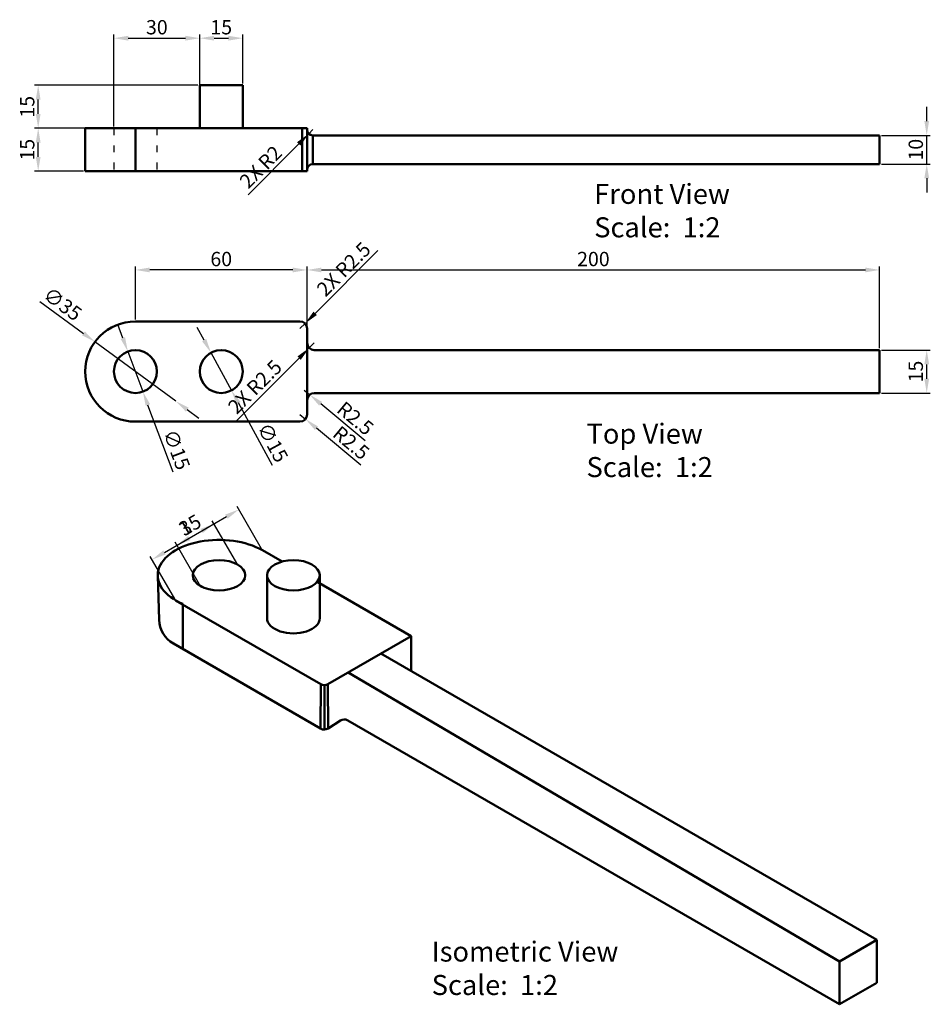
# Model space of a CAD drawing. Units: millimetres. Extents: x 2577 to 3382, y -259 to 299.
# Tile 2 of 2: x 3064 to 3382, y -124 to 220. Entities that reach past the tile are written whole.
import ezdxf

# ---------------------------------------------------------------- set-up
doc = ezdxf.new("R2010")
doc.units = ezdxf.units.MM
doc.linetypes.add('ACAD_ISO03W100', pattern=[30, 12, -18])
for name, color, linetype, lineweight in [('M-DIMS', 2, 'Continuous', 25), ('M-HIDN', 7, 'ACAD_ISO03W100', 25), ('M-OUTL', 7, 'Continuous', 50), ('M-TEXT', 7, 'Continuous', 25)]:
    doc.layers.add(name, color=color, linetype=linetype, lineweight=lineweight)
doc.styles.get("Standard").update_dxf_attribs({"font": 'arial.ttf'})
doc.dimstyles.new('ISO-25', dxfattribs={"dimtxt": 5, "dimasz": 5, "dimexe": 1.25, "dimexo": 0.625, "dimtad": 1, "dimdec": 0, "dimtxsty": 'Standard', "dimcen": 2.5, "dimadec": 0, "dimazin": 0, "dimtfac": 1, "dimtdec": 0, "dimtmove": 0, "dimatfit": 3, "dimfxl": 1, "dimarcsym": 0})

# ---------------------------------------------------------------- blocks, each defined once
blk = doc.blocks.new('*D12')
at = {"layer": 'Defpoints', "color": 0, "transparency": 16777216}
for p in [(3090.35, 107.42), (3118.56, 86.7)]:
    blk.add_point(p, dxfattribs=at)
at = {"layer": 'M-DIMS', "color": 0, "lineweight": -2, "transparency": 16777216}
for p, q in [((3071.1, 121.56), (3086.32, 110.38)), ((3118.56, 86.7), (3090.35, 107.42)), ((3122.59, 83.74), (3126.62, 80.78))]:
    blk.add_line(p, q, dxfattribs=at)
at = {"layer": 'M-DIMS', "color": 0, "transparency": 16777216}
for points in [[(3086.81, 111.05), (3085.83, 109.71), (3090.35, 107.42)], [(3123.08, 84.41), (3122.1, 83.07), (3118.56, 86.7)]]:
    blk.add_solid(points, dxfattribs=at)
at = {"layer": 'M-DIMS', "color": 0, "transparency": 16777216, "insert": (3078.66, 120.12), "char_height": 5, "attachment_point": 5, "rotation": 323.7034}
blk.add_mtext('∅35', dxfattribs=at)
blk = doc.blocks.new('*D13')
at = {"layer": 'Defpoints', "color": 0, "transparency": 16777216}
for p in [(3101.83, 104.08), (3107.08, 90.03)]:
    blk.add_point(p, dxfattribs=at)
at = {"layer": 'M-DIMS', "color": 0, "lineweight": -2, "transparency": 16777216}
for p, q in [((3100.07, 108.76), (3098.32, 113.45)), ((3101.83, 104.08), (3107.08, 90.03)), ((3117.62, 61.88), (3108.84, 85.35))]:
    blk.add_line(p, q, dxfattribs=at)
at = {"layer": 'M-DIMS', "color": 0, "transparency": 16777216}
for points in [[(3100.85, 109.06), (3099.29, 108.47), (3101.83, 104.08)], [(3109.62, 85.64), (3108.06, 85.06), (3107.08, 90.03)]]:
    blk.add_solid(points, dxfattribs=at)
at = {"layer": 'M-DIMS', "color": 0, "transparency": 16777216, "insert": (3118.29, 69.55), "char_height": 5, "attachment_point": 5, "rotation": 290.5206}
blk.add_mtext('∅15', dxfattribs=at)
blk = doc.blocks.new('*D14')
at = {"layer": 'Defpoints', "color": 0, "transparency": 16777216}
for p in [(3130.87, 103.65), (3138.04, 90.47)]:
    blk.add_point(p, dxfattribs=at)
at = {"layer": 'M-DIMS', "color": 0, "lineweight": -2, "transparency": 16777216}
for p, q in [((3128.48, 108.04), (3126.09, 112.43)), ((3130.87, 103.65), (3138.04, 90.47)), ((3152.31, 64.25), (3140.43, 86.08))]:
    blk.add_line(p, q, dxfattribs=at)
at = {"layer": 'M-DIMS', "color": 0, "transparency": 16777216}
for points in [[(3129.21, 108.44), (3127.75, 107.64), (3130.87, 103.65)], [(3141.16, 86.48), (3139.7, 85.68), (3138.04, 90.47)]]:
    blk.add_solid(points, dxfattribs=at)
at = {"layer": 'M-DIMS', "color": 0, "transparency": 16777216, "insert": (3151.9, 71.93), "char_height": 5, "attachment_point": 5, "rotation": 298.5506}
blk.add_mtext('∅15', dxfattribs=at)
blk = doc.blocks.new('*D15')
at = {"layer": 'Defpoints', "color": 0, "transparency": 16777216}
for p in [(3161.96, 82.06), (3163.88, 80.46)]:
    blk.add_point(p, dxfattribs=at)
at = {"layer": 'M-DIMS', "color": 0, "lineweight": -2, "transparency": 16777216}
for p, q in [((3161.96, 82.06), (3163.88, 80.46)), ((3183.23, 64.36), (3167.72, 77.26))]:
    blk.add_line(p, q, dxfattribs=at)
at = {"layer": 'M-DIMS', "color": 0, "transparency": 16777216}
blk.add_solid([(3168.25, 77.9), (3167.19, 76.62), (3163.88, 80.46)], dxfattribs=at)
at = {"layer": 'M-DIMS', "color": 0, "transparency": 16777216, "insert": (3179.43, 71.66), "char_height": 5, "attachment_point": 5, "rotation": 320.2486}
blk.add_mtext('R2.5', dxfattribs=at)
blk = doc.blocks.new('*D16')
at = {"layer": 'Defpoints', "color": 0, "transparency": 16777216}
for p in [(3163.42, 90.59), (3165.34, 88.99)]:
    blk.add_point(p, dxfattribs=at)
at = {"layer": 'M-DIMS', "color": 0, "lineweight": -2, "transparency": 16777216}
for p, q in [((3163.42, 90.59), (3165.34, 88.99)), ((3184.7, 72.9), (3169.19, 85.8))]:
    blk.add_line(p, q, dxfattribs=at)
at = {"layer": 'M-DIMS', "color": 0, "transparency": 16777216}
blk.add_solid([(3169.72, 86.44), (3168.65, 85.16), (3165.34, 88.99)], dxfattribs=at)
at = {"layer": 'M-DIMS', "color": 0, "transparency": 16777216, "insert": (3180.9, 80.19), "char_height": 5, "attachment_point": 5, "rotation": 320.2486}
blk.add_mtext('R2.5', dxfattribs=at)
blk = doc.blocks.new('*D17')
at = {"layer": 'Defpoints', "color": 0, "transparency": 16777216}
for p in [(3364.46, 132.54), (3164.46, 107.06), (3364.46, 104.56)]:
    blk.add_point(p, dxfattribs=at)
at = {"layer": 'M-DIMS', "color": 0, "lineweight": -2, "transparency": 16777216}
for p, q in [((3164.46, 107.68), (3164.46, 133.79)), ((3169.46, 132.54), (3359.46, 132.54)), ((3364.46, 105.18), (3364.46, 133.79))]:
    blk.add_line(p, q, dxfattribs=at)
at = {"layer": 'M-DIMS', "color": 0, "transparency": 16777216}
for points in [[(3169.46, 133.37), (3169.46, 131.7), (3164.46, 132.54)], [(3359.46, 133.37), (3359.46, 131.7), (3364.46, 132.54)]]:
    blk.add_solid(points, dxfattribs=at)
at = {"layer": 'M-DIMS', "color": 0, "transparency": 16777216, "insert": (3264.46, 135.71), "char_height": 5, "attachment_point": 5}
blk.add_mtext('200', dxfattribs=at)
blk = doc.blocks.new('*D18')
at = {"layer": 'Defpoints', "color": 0, "transparency": 16777216}
for p in [(3104.46, 132.54), (3104.46, 114.56), (3164.44, 112.32)]:
    blk.add_point(p, dxfattribs=at)
at = {"layer": 'M-DIMS', "color": 0, "lineweight": -2, "transparency": 16777216}
for p, q in [((3104.46, 115.18), (3104.46, 133.79)), ((3159.44, 132.54), (3109.46, 132.54)), ((3164.44, 112.94), (3164.44, 133.79))]:
    blk.add_line(p, q, dxfattribs=at)
at = {"layer": 'M-DIMS', "color": 0, "transparency": 16777216}
for points in [[(3109.46, 133.37), (3109.46, 131.7), (3104.46, 132.54)], [(3159.44, 133.37), (3159.44, 131.7), (3164.44, 132.54)]]:
    blk.add_solid(points, dxfattribs=at)
at = {"layer": 'M-DIMS', "color": 0, "transparency": 16777216, "insert": (3134.45, 135.71), "char_height": 5, "attachment_point": 5}
blk.add_mtext('60', dxfattribs=at)
blk = doc.blocks.new('BORE-D15-TOP')
blk.add_circle((0, 0), 7.5)
blk = doc.blocks.new('BORE-D15-ISO')
blk.add_ellipse((0, 0), major_axis=(-9.19, 0), ratio=0.57735)
blk = doc.blocks.new('PIN-D15-TOP')
blk.add_circle((0, 0), 7.5)
blk = doc.blocks.new('*D28')
at = {"layer": 'Defpoints', "color": 0, "transparency": 16777216}
for p in [(3070.51, 182.05), (3086.96, 182.05), (3086.96, 167.05)]:
    blk.add_point(p, dxfattribs=at)
at = {"layer": 'M-DIMS', "color": 0, "lineweight": -2, "transparency": 16777216}
for p, q in [((3086.33, 182.05), (3069.26, 182.05)), ((3070.51, 172.05), (3070.51, 177.05)), ((3086.33, 167.05), (3069.26, 167.05))]:
    blk.add_line(p, q, dxfattribs=at)
at = {"layer": 'M-DIMS', "color": 0, "transparency": 16777216}
for points in [[(3069.67, 177.05), (3071.34, 177.05), (3070.51, 182.05)], [(3069.67, 172.05), (3071.34, 172.05), (3070.51, 167.05)]]:
    blk.add_solid(points, dxfattribs=at)
at = {"layer": 'M-DIMS', "color": 0, "transparency": 16777216, "insert": (3067.33, 174.55), "char_height": 5, "attachment_point": 5, "rotation": 90}
blk.add_mtext('15', dxfattribs=at)
blk = doc.blocks.new('*D29')
at = {"layer": 'Defpoints', "color": 0, "transparency": 16777216}
for p in [(3070.51, 197.05), (3126.96, 197.05), (3126.96, 182.05)]:
    blk.add_point(p, dxfattribs=at)
at = {"layer": 'M-DIMS', "color": 0, "lineweight": -2, "transparency": 16777216}
for p, q in [((3126.33, 197.05), (3069.26, 197.05)), ((3070.51, 187.05), (3070.51, 192.05)), ((3126.33, 182.05), (3069.26, 182.05))]:
    blk.add_line(p, q, dxfattribs=at)
at = {"layer": 'M-DIMS', "color": 0, "transparency": 16777216}
for points in [[(3069.67, 192.05), (3071.34, 192.05), (3070.51, 197.05)], [(3069.67, 187.05), (3071.34, 187.05), (3070.51, 182.05)]]:
    blk.add_solid(points, dxfattribs=at)
at = {"layer": 'M-DIMS', "color": 0, "transparency": 16777216, "insert": (3067.33, 189.55), "char_height": 5, "attachment_point": 5, "rotation": 90}
blk.add_mtext('15', dxfattribs=at)
blk = doc.blocks.new('*D30')
at = {"layer": 'Defpoints', "color": 0, "transparency": 16777216}
for p in [(3364.46, 179.55), (3380.91, 179.55), (3364.46, 169.55)]:
    blk.add_point(p, dxfattribs=at)
at = {"layer": 'M-DIMS', "color": 0, "lineweight": -2, "transparency": 16777216}
for p, q in [((3380.91, 184.55), (3380.91, 189.55)), ((3365.08, 179.55), (3382.16, 179.55)), ((3380.91, 169.55), (3380.91, 179.55)), ((3365.08, 169.55), (3382.16, 169.55)), ((3380.91, 164.55), (3380.91, 159.55))]:
    blk.add_line(p, q, dxfattribs=at)
at = {"layer": 'M-DIMS', "color": 0, "transparency": 16777216}
for points in [[(3380.07, 184.55), (3381.74, 184.55), (3380.91, 179.55)], [(3380.07, 164.55), (3381.74, 164.55), (3380.91, 169.55)]]:
    blk.add_solid(points, dxfattribs=at)
at = {"layer": 'M-DIMS', "color": 0, "transparency": 16777216, "insert": (3377.73, 174.55), "char_height": 5, "attachment_point": 5, "rotation": 90}
blk.add_mtext('10', dxfattribs=at)
blk = doc.blocks.new('*D31')
at = {"layer": 'Defpoints', "color": 0, "transparency": 16777216}
for p in [(3364.46, 104.56), (3380.91, 104.56), (3364.46, 89.56)]:
    blk.add_point(p, dxfattribs=at)
at = {"layer": 'M-DIMS', "color": 0, "lineweight": -2, "transparency": 16777216}
for p, q in [((3365.08, 104.56), (3382.16, 104.56)), ((3380.91, 94.56), (3380.91, 99.56)), ((3365.08, 89.56), (3382.16, 89.56))]:
    blk.add_line(p, q, dxfattribs=at)
at = {"layer": 'M-DIMS', "color": 0, "transparency": 16777216}
for points in [[(3380.07, 99.56), (3381.74, 99.56), (3380.91, 104.56)], [(3380.07, 94.56), (3381.74, 94.56), (3380.91, 89.56)]]:
    blk.add_solid(points, dxfattribs=at)
at = {"layer": 'M-DIMS', "color": 0, "transparency": 16777216, "insert": (3377.73, 97.06), "char_height": 5, "attachment_point": 5, "rotation": 90}
blk.add_mtext('15', dxfattribs=at)
blk = doc.blocks.new('*D32')
at = {"layer": 'Defpoints', "color": 0, "transparency": 16777216}
for p in [(3126.96, 213.5), (3096.96, 182.05), (3126.96, 182.05)]:
    blk.add_point(p, dxfattribs=at)
at = {"layer": 'M-DIMS', "color": 0, "lineweight": -2, "transparency": 16777216}
for p, q in [((3096.96, 182.67), (3096.96, 214.75)), ((3101.96, 213.5), (3121.96, 213.5)), ((3126.96, 182.67), (3126.96, 214.75))]:
    blk.add_line(p, q, dxfattribs=at)
at = {"layer": 'M-DIMS', "color": 0, "transparency": 16777216}
for points in [[(3101.96, 214.33), (3101.96, 212.66), (3096.96, 213.5)], [(3121.96, 214.33), (3121.96, 212.66), (3126.96, 213.5)]]:
    blk.add_solid(points, dxfattribs=at)
at = {"layer": 'M-DIMS', "color": 0, "transparency": 16777216, "insert": (3111.96, 216.68), "char_height": 5, "attachment_point": 5}
blk.add_mtext('30', dxfattribs=at)
blk = doc.blocks.new('*D33')
at = {"layer": 'Defpoints', "color": 0, "transparency": 16777216}
for p in [(3140.61, 48.87), (3148.83, 34.63), (3118.52, 17.13)]:
    blk.add_point(p, dxfattribs=at)
at = {"layer": 'M-DIMS', "color": 0, "lineweight": -2, "transparency": 16777216}
for p, q in [((3148.52, 35.17), (3139.98, 49.95)), ((3114.63, 33.87), (3136.28, 46.37)), ((3118.21, 17.67), (3109.67, 32.45))]:
    blk.add_line(p, q, dxfattribs=at)
at = {"layer": 'M-DIMS', "color": 0, "transparency": 16777216}
for points in [[(3135.86, 47.09), (3136.69, 45.65), (3140.61, 48.87)], [(3114.21, 34.59), (3115.04, 33.15), (3110.3, 31.37)]]:
    blk.add_solid(points, dxfattribs=at)
at = {"layer": 'M-DIMS', "color": 0, "transparency": 16777216, "insert": (3123.86, 42.88), "char_height": 5, "attachment_point": 5, "rotation": 30}
blk.add_mtext('35', dxfattribs=at)
blk = doc.blocks.new('*D34')
at = {"layer": 'Defpoints', "color": 0, "transparency": 16777216}
for p in [(3131.95, 43.87), (3140.17, 29.63), (3127.18, 22.13)]:
    blk.add_point(p, dxfattribs=at)
at = {"layer": 'M-DIMS', "color": 0, "lineweight": -2, "transparency": 16777216}
for p, q in [((3139.86, 30.17), (3131.32, 44.95)), ((3123.29, 38.87), (3127.62, 41.37)), ((3126.87, 22.67), (3118.33, 37.45))]:
    blk.add_line(p, q, dxfattribs=at)
at = {"layer": 'M-DIMS', "color": 0, "transparency": 16777216}
for points in [[(3127.2, 42.09), (3128.03, 40.65), (3131.95, 43.87)], [(3122.87, 39.59), (3123.7, 38.15), (3118.96, 36.37)]]:
    blk.add_solid(points, dxfattribs=at)
at = {"layer": 'M-DIMS', "color": 0, "transparency": 16777216, "insert": (3123.86, 42.87), "char_height": 5, "attachment_point": 5, "rotation": 30}
blk.add_mtext('15', dxfattribs=at)
blk = doc.blocks.new('*D35')
at = {"layer": 'Defpoints', "color": 0, "transparency": 16777216}
for p in [(3141.96, 213.5), (3126.96, 197.05), (3141.96, 197.05)]:
    blk.add_point(p, dxfattribs=at)
at = {"layer": 'M-DIMS', "color": 0, "lineweight": -2, "transparency": 16777216}
for p, q in [((3126.96, 197.67), (3126.96, 214.75)), ((3131.96, 213.5), (3136.96, 213.5)), ((3141.96, 197.67), (3141.96, 214.75))]:
    blk.add_line(p, q, dxfattribs=at)
at = {"layer": 'M-DIMS', "color": 0, "transparency": 16777216}
for points in [[(3131.96, 214.33), (3131.96, 212.66), (3126.96, 213.5)], [(3136.96, 214.33), (3136.96, 212.66), (3141.96, 213.5)]]:
    blk.add_solid(points, dxfattribs=at)
at = {"layer": 'M-DIMS', "color": 0, "transparency": 16777216, "insert": (3134.46, 216.68), "char_height": 5, "attachment_point": 5}
blk.add_mtext('15', dxfattribs=at)
blk = doc.blocks.new('*D41')
at = {"layer": 'Defpoints', "color": 0, "transparency": 16777216}
for p in [(3166.96, 107.06), (3165.19, 105.29)]:
    blk.add_point(p, dxfattribs=at)
at = {"layer": 'M-DIMS', "color": 0, "lineweight": -2, "transparency": 16777216}
for p, q in [((3166.96, 107.06), (3165.19, 105.29)), ((3139.74, 79.82), (3161.66, 101.75))]:
    blk.add_line(p, q, dxfattribs=at)
at = {"layer": 'M-DIMS', "color": 0, "transparency": 16777216}
blk.add_solid([(3161.07, 102.34), (3162.24, 101.16), (3165.19, 105.29)], dxfattribs=at)
at = {"layer": 'M-DIMS', "color": 0, "transparency": 16777216, "insert": (3146.68, 91.26), "char_height": 5, "attachment_point": 5, "rotation": 45.0321}
blk.add_mtext('2X R2.5', dxfattribs=at)
blk = doc.blocks.new('*D42')
at = {"layer": 'Defpoints', "color": 0, "transparency": 16777216}
for p in [(3163.72, 113.83), (3161.96, 112.06)]:
    blk.add_point(p, dxfattribs=at)
at = {"layer": 'M-DIMS', "color": 0, "lineweight": -2, "transparency": 16777216}
for p, q in [((3189.12, 139.35), (3167.25, 117.37)), ((3161.96, 112.06), (3163.72, 113.83))]:
    blk.add_line(p, q, dxfattribs=at)
at = {"layer": 'M-DIMS', "color": 0, "transparency": 16777216}
blk.add_solid([(3166.66, 117.96), (3167.84, 116.79), (3163.72, 113.83)], dxfattribs=at)
at = {"layer": 'M-DIMS', "color": 0, "transparency": 16777216, "insert": (3177.7, 132.37), "char_height": 5, "attachment_point": 5, "rotation": 45.13}
blk.add_mtext('2X R2.5', dxfattribs=at)
blk = doc.blocks.new('*D43')
at = {"layer": 'Defpoints', "color": 0, "transparency": 16777216}
for p in [(3165.04, 180.13), (3166.44, 181.55)]:
    blk.add_point(p, dxfattribs=at)
at = {"layer": 'M-DIMS', "color": 0, "lineweight": -2, "transparency": 16777216}
for p, q in [((3166.44, 181.55), (3165.04, 180.13)), ((3143.87, 158.73), (3161.52, 176.57))]:
    blk.add_line(p, q, dxfattribs=at)
at = {"layer": 'M-DIMS', "color": 0, "transparency": 16777216}
blk.add_solid([(3160.93, 177.16), (3162.11, 175.98), (3165.04, 180.13)], dxfattribs=at)
at = {"layer": 'M-DIMS', "color": 0, "transparency": 16777216, "insert": (3148.71, 168.08), "char_height": 5, "attachment_point": 5, "rotation": 45.3115}
blk.add_mtext('2X R2', dxfattribs=at)

msp = doc.modelspace()

# ---------------------------------------------------------------- linework, layer by layer
at = {"layer": 'M-HIDN', "ltscale": 0.2}
for p, q in [((3096.96, 182.05), (3096.96, 167.05)), ((3111.96, 182.05), (3111.96, 167.05))]:
    msp.add_line(p, q, dxfattribs=at)
at = {"layer": 'M-OUTL'}
for p, q in [((3141.96, 197.05), (3126.96, 197.05)), ((3126.96, 197.05), (3126.96, 182.05)), ((3141.96, 182.05), (3141.96, 197.05)), ((3086.96, 182.05), (3086.96, 167.05)), ((3164.44, 182.05), (3086.96, 182.05)), ((3104.46, 182.05), (3104.46, 167.05)), ((3162.77, 167.05), (3162.77, 182.05)), ((3164.44, 181.55), (3164.44, 182.05)), ((3164.44, 167.05), (3164.44, 181.55)), ((3166.44, 179.55), (3364.46, 179.55)), ((3166.44, 169.55), (3166.44, 179.55)), ((3364.46, 169.55), (3364.46, 179.55)), ((3364.46, 169.55), (3166.44, 169.55)), ((3164.44, 167.05), (3086.96, 167.05)), ((3164.44, 167.05), (3164.44, 167.55)), ((3104.46, 114.56), (3161.96, 114.56)), ((3164.46, 112.06), (3164.46, 107.06)), ((3164.46, 112.06), (3164.46, 87.06)), ((3364.46, 104.56), (3166.96, 104.56)), ((3166.96, 104.56), (3364.46, 104.56)), ((3364.46, 104.56), (3364.46, 89.56)), ((3364.46, 104.56), (3364.46, 89.56)), ((3364.46, 89.56), (3166.96, 89.56)), ((3164.46, 82.06), (3164.46, 87.06)), ((3104.46, 79.56), (3161.96, 79.56)), ((3148.83, 34.63), (3155.7, 30.66)), ((3112.74, 10.34), (3112.25, 25.65)), ((3150.47, 10.88), (3150.47, 25.88)), ((3168.84, 10.88), (3168.84, 25.88)), ((3126.18, 22.81), (3128.24, 21.6)), ((3167.95, 23.59), (3200.79, 4.63)), ((3118.52, 17.13), (3169.23, -12.15)), ((3121.05, 15.88), (3121.05, 0.09)), ((3171.73, -12.15), (3200.79, 4.63)), ((3200.79, 4.63), (3200.79, -7.57)), ((3117.74, 2.01), (3169.16, -27.68)), ((3190.23, -1.47), (3363.44, -101.47)), ((3178.77, -8.09), (3350.45, -108.97)), ((3169.23, -12.15), (3169.16, -27.68)), ((3170.48, -12.49), (3170.48, -28.06)), ((3171.73, -12.15), (3171.76, -27.62)), ((3176.06, -24.86), (3171.76, -27.62)), ((3350.45, -123.97), (3178.66, -24.79)), ((3363.44, -101.47), (3350.45, -108.97)), ((3363.44, -116.47), (3363.44, -101.47)), ((3350.45, -108.97), (3350.45, -123.97)), ((3350.45, -123.97), (3363.44, -116.47))]:
    msp.add_line(p, q, dxfattribs=at)
for centre, radius, start, end in [((3166.44, 181.55), 2, 180, 270), ((3166.44, 167.55), 2, 90, 180), ((3104.46, 97.06), 17.5, 90, 270), ((3161.96, 112.06), 2.5, 0, 90), ((3166.96, 107.06), 2.5, 180, 270), ((3166.96, 87.06), 2.5, 90, 180), ((3161.96, 82.06), 2.5, 270, 0), ((3122.74, 10.67), 10, 181.8505, 240), ((3170.48, -9.99), 2.5, 240, 300), ((3177.41, -26.96), 2.5, 60, 122.7566), ((3170.41, -25.52), 2.5, 240, 302.7566)]:
    msp.add_arc(centre, radius, start, end, dxfattribs=at)
for centre, major_axis, start_param, end_param in [((3133.68, 25.88), (-21.43, 0), 3.926991, 7.224142), ((3133.68, 5.88), (-21.43, 0), 5.342229, 5.35444), ((3159.66, 10.88), (-9.19, 0), 0, 3.141593)]:
    msp.add_ellipse(centre, major_axis=major_axis, ratio=0.57735, start_param=start_param, end_param=end_param, dxfattribs=at)
msp.add_ellipse((3159.66, 25.88), major_axis=(-9.19, 0), ratio=0.57735, dxfattribs=at)

# ---------------------------------------------------------------- block references
for name, p in [('BORE-D15-TOP', (3104.46, 97.06)), ('PIN-D15-TOP', (3134.46, 97.06)), ('BORE-D15-ISO', (3133.68, 25.88))]:
    msp.add_blockref(name, p, dxfattribs=at)

# ---------------------------------------------------------------- texts
at = {"layer": 'M-TEXT', "char_height": 7, "attachment_point": 1}
for s, insert in [('Front View\\PScale:  1:2', (3264.74, 162.6)), ('Top View\\PScale:  1:2', (3262.05, 78.85)), ('Isometric View\\PScale:  1:2', (3207.97, -102.05))]:
    msp.add_mtext_dynamic_manual_height_columns(s, width=128.7125, gutter_width=12.5, heights=[0], dxfattribs=dict(at, insert=insert))

# ---------------------------------------------------------------- dimensions: what is measured, and where the dimension line sits
at = {"layer": 'M-DIMS'}
for base, p1, p2, override, picture, middle in [((3126.96, 213.5), (3096.96, 182.05), (3126.96, 182.05), {"dimdec": 0, "dimlfac": 1, "dimrnd": 0, "dimzin": 0, "dimdsep": 46, "dimlunit": 2}, '*D32', (3111.96, 216.68)), ((3141.96, 213.5), (3126.96, 197.05), (3141.96, 197.05), {"dimdec": 0, "dimlfac": 1, "dimrnd": 0, "dimzin": 0, "dimdsep": 46, "dimlunit": 2}, '*D35', (3134.46, 216.68)), ((3104.46, 132.54), (3164.44, 112.32), (3104.46, 114.56), {"dimclrd": 0, "dimclre": 0, "dimclrt": 0}, '*D18', (3134.45, 135.71)), ((3364.46, 132.54), (3164.46, 107.06), (3364.46, 104.56), {"dimclrd": 0, "dimclre": 0, "dimclrt": 0}, '*D17', (3264.46, 135.71))]:
    dim = msp.add_linear_dim(base=base, p1=p1, p2=p2, dimstyle='ISO-25', override=override, dxfattribs=at)
    dim.commit()
    dim.dimension.update_dxf_attribs({"geometry": picture, "text_midpoint": middle})
for base, p1, p2, angle, picture, middle in [((3070.51, 197.05), (3126.96, 182.05), (3126.96, 197.05), 90, '*D29', (3067.33, 189.55)), ((3380.91, 179.55), (3364.46, 169.55), (3364.46, 179.55), 90, '*D30', (3377.73, 174.55)), ((3070.51, 182.05), (3086.96, 167.05), (3086.96, 182.05), 90, '*D28', (3067.33, 174.55)), ((3380.91, 104.56), (3364.46, 89.56), (3364.46, 104.56), 90, '*D31', (3377.73, 97.06)), ((3140.61, 48.87), (3118.52, 17.13), (3148.83, 34.63), 30, '*D33', (3123.86, 42.88)), ((3131.95, 43.87), (3127.18, 22.13), (3140.17, 29.63), 30, '*D34', (3123.86, 42.87))]:
    dim = msp.add_linear_dim(base=base, p1=p1, p2=p2, angle=angle, dimstyle='ISO-25', override={"dimdec": 0, "dimlfac": 1, "dimrnd": 0, "dimzin": 0, "dimdsep": 46, "dimlunit": 2}, dxfattribs=at)
    dim.commit()
    dim.dimension.update_dxf_attribs({"geometry": picture, "text_midpoint": middle})
for center, mpoint, text, override, picture, middle in [((3166.44, 181.55), (3165.04, 180.13), '2X <>', {"dimdec": 0, "dimlfac": 1, "dimrnd": 0, "dimzin": 0, "dimdsep": 46, "dimlunit": 2}, '*D43', (3148.71, 168.08)), ((3161.96, 112.06), (3163.72, 113.83), '2X <>', {"dimdec": 1, "dimlfac": 1, "dimrnd": 0, "dimzin": 0, "dimdsep": 46, "dimlunit": 2}, '*D42', (3177.7, 132.37)), ((3166.96, 107.06), (3165.19, 105.29), '2X <>', {"dimdec": 1, "dimlfac": 1, "dimrnd": 0, "dimzin": 0, "dimdsep": 46, "dimlunit": 2}, '*D41', (3146.68, 91.26)), ((3163.42, 90.59), (3165.34, 88.99), 'R2.5', {"dimclrd": 0, "dimclre": 0, "dimclrt": 0}, '*D16', (3180.9, 80.19)), ((3161.96, 82.06), (3163.88, 80.46), 'R2.5', {"dimclrd": 0, "dimclre": 0, "dimclrt": 0}, '*D15', (3179.43, 71.66))]:
    dim = msp.add_radius_dim(center=center, mpoint=mpoint, text=text, dimstyle='ISO-25', override=override, dxfattribs=at)
    dim.commit()
    dim.dimension.update_dxf_attribs({"geometry": picture, "text_midpoint": middle})
dim = msp.add_diameter_dim_2p(p1=(3118.56, 86.7), p2=(3090.35, 107.42), dimstyle='ISO-25', override={"dimclrd": 0, "dimclre": 0, "dimclrt": 0}, dxfattribs=at)
dim.commit()
dim.dimension.update_dxf_attribs({"geometry": '*D12', "text_midpoint": (3078.66, 120.12)})
for p1, p2, picture, middle in [((3101.83, 104.08), (3107.08, 90.03), '*D13', (3115.19, 68.39)), ((3130.87, 103.65), (3138.04, 90.47), '*D14', (3148.99, 70.35))]:
    dim = msp.add_diameter_dim_2p(p1=p1, p2=p2, dimstyle='ISO-25', override={"dimclrd": 0, "dimclre": 0, "dimclrt": 0}, dxfattribs=at)
    dim.commit()
    dim.dimension.update_dxf_attribs({"geometry": picture, "text_midpoint": middle, "dimtype": 163})

doc.saveas('drawing.dxf')
